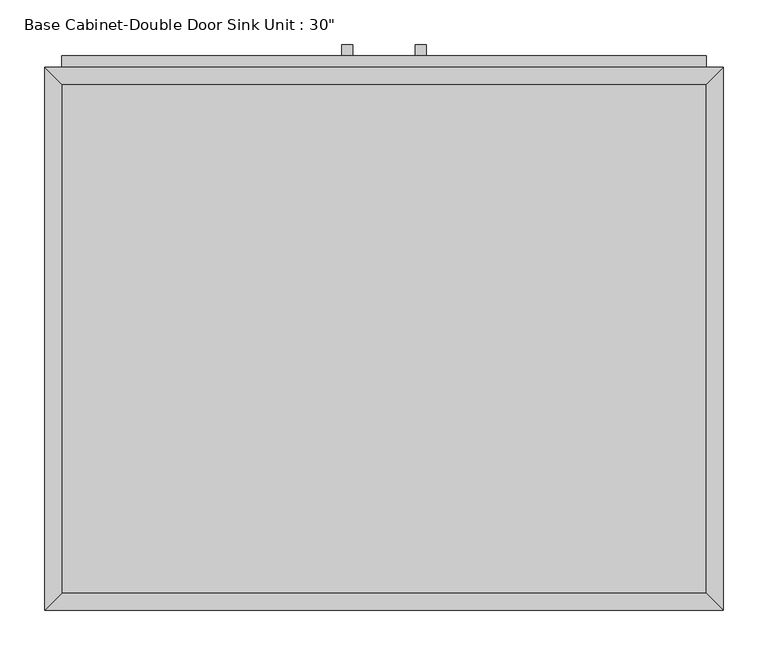
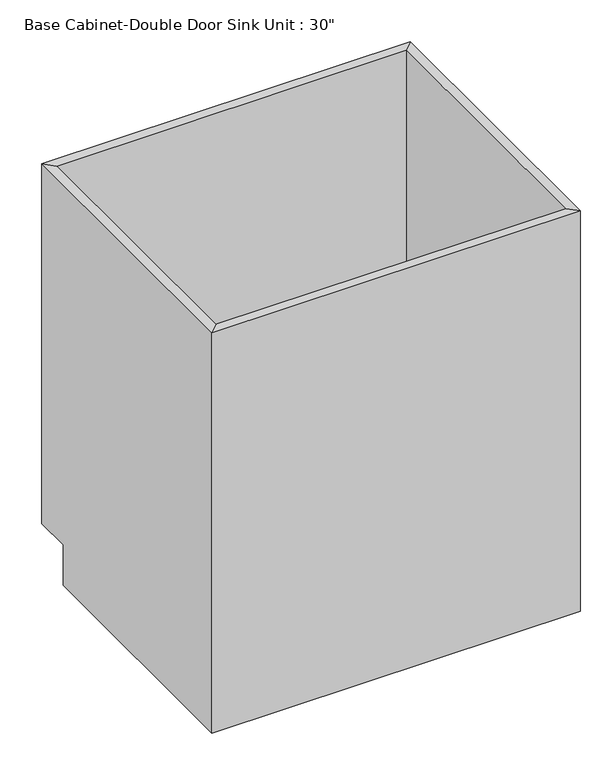
"""IFC4 building model written with IfcOpenShell, lengths in millimetres: furniture geometry."""

from ifc_helpers import new_model, si_unit, frame, origin, place, context, project, spatial, polyline, outline, extrude, faceted_brep, source, transform, mapped, element, save


def furniture_2feb49e6(model_context):
    return source(origin(), model_context, "Body", "SolidModel", [
        faceted_brep([(380.6877049, 590.55, 876.3), (-343.2122951, 590.55, 876.3), (-343.2122951, 590.55, 88.9), (380.6877049, 590.55, 88.9), (399.7377049, 609.6, 876.3), (-362.2622951, 609.6, 876.3), (399.7377049, 609.6, 88.9), (-362.2622951, 609.6, 88.9), (-343.2122951, 19.05, 876.3), (-343.2122951, 19.05, 88.9), (-343.2122951, 533.4, 88.9), (-362.2622951, 0.0, 876.3), (-362.2622951, 533.4, 88.9), (-362.2622951, 533.4, 0.0), (-362.2622951, 0.0, 0.0), (380.6877049, 19.05, 876.3), (380.6877049, 19.05, 88.9), (399.7377049, 0.0, 876.3), (399.7377049, 0.0, 0.0), (380.6877049, 533.4, 88.9), (399.7377049, 533.4, 0.0), (399.7377049, 533.4, 88.9)], [[[0, 1, 2, 3]], [[0, 4, 5, 1]], [[4, 6, 7, 5]], [[2, 7, 6, 3]], [[1, 8, 9, 10, 2]], [[5, 11, 8, 1]], [[7, 12, 13, 14, 11, 5]], [[2, 10, 12, 7]], [[8, 15, 16, 9]], [[11, 17, 15, 8]], [[14, 18, 17, 11]], [[3, 19, 16, 15, 0]], [[0, 15, 17, 4]], [[4, 17, 18, 20, 21, 6]], [[6, 21, 19, 3]], [[10, 9, 16, 19]], [[18, 14, 13, 20]], [[13, 12, 10, 19, 21, 20]]]),
        extrude(outline(polyline([(-16.1872951, 635.0), (-16.1872951, 622.3), (-28.8872951, 622.3), (-28.8872951, 635.0), (-16.1872951, 635.0)])), frame((0.0, 0.0, 573.769895), z_axis=(0.0, 0.0, 1.0), x_axis=(1.0, 0.0, 0.0)), (0.0, 0.0, 1.0), 124.730105),
        extrude(outline(polyline([(66.3627049, 635.0), (66.3627049, 622.3), (53.6627049, 622.3), (53.6627049, 635.0), (66.3627049, 635.0)])), frame((0.0, 0.0, 573.769895), z_axis=(0.0, 0.0, 1.0), x_axis=(1.0, 0.0, 0.0)), (0.0, 0.0, 1.0), 124.730105),
        extrude(outline(polyline([(380.6877049, 19.05), (-343.2122951, 19.05), (-343.2122951, 590.55), (380.6877049, 590.55), (380.6877049, 19.05)])), frame((0.0, 0.0, 88.9), z_axis=(0.0, 0.0, 1.0), x_axis=(1.0, 0.0, 0.0)), (0.0, 0.0, 1.0), 19.05),
        extrude(outline(polyline([(9.2127049, 622.3), (9.2127049, 609.6), (-343.2122951, 609.6), (-343.2122951, 622.3), (9.2127049, 622.3)])), frame((0.0, 0.0, 107.95), z_axis=(0.0, 0.0, 1.0), x_axis=(1.0, 0.0, 0.0)), (0.0, 0.0, 1.0), 628.65),
        extrude(outline(polyline([(380.6877049, 622.3), (380.6877049, 609.6), (28.2627049, 609.6), (28.2627049, 622.3), (380.6877049, 622.3)])), frame((0.0, 0.0, 107.95), z_axis=(0.0, 0.0, 1.0), x_axis=(1.0, 0.0, 0.0)), (0.0, 0.0, 1.0), 628.65),
        extrude(outline(polyline([(380.6877049, 622.3), (380.6877049, 609.6), (-343.2122951, 609.6), (-343.2122951, 622.3), (380.6877049, 622.3)])), frame((0.0, 0.0, 755.65), z_axis=(0.0, 0.0, 1.0), x_axis=(1.0, 0.0, 0.0)), (0.0, 0.0, 1.0), 101.6),
    ])


if __name__ == "__main__":
    model = new_model("IFC4")
    model_context = context("Model", 3, world=origin())
    ifc_project = project(units=[si_unit("LENGTHUNIT", "METRE", prefix="MILLI")], contexts=[model_context])
    site = spatial("IfcSite", under=ifc_project)
    building = spatial("IfcBuilding", under=site)
    placement = place(None, origin())
    furniture_shape = furniture_2feb49e6(model_context)
    element("IfcFurniture", 1, ObjectType="Base Cabinet-Double Door Sink Unit : 30\"", at=placement, inside=building, context=model_context, shape_type="MappedRepresentation", body=[
        mapped(furniture_shape, transform((0.0, 0.0, 0.0), x_axis=(1.0, 0.0, 0.0), y_axis=(0.0, 1.0, 0.0), z_axis=(0.0, 0.0, 1.0))),
    ])
    save(model, "model.ifc")

# Revit data of these elements
# Type "Base Cabinet-Double Door Sink Unit : 30\""
#   Assembly Code = "C1030410"
#   Depth = 2' - 0"
#   Height = 2' - 10 1/2"
#   Toe Depth = 0' - 3"
#   Toe Height = 0' - 3 1/2"
#   Width = 2' - 6"
#   Cabinet Material = none
#   Door/Drawer Material = none
#   Handle Material = Cabinets - Handles
#   Default Elevation = 0
# Element 1 (IfcFurniture, "Base Cabinet-Double Door Sink Unit : 30\"")
#   Materials on its faces: "Cabinets", "Cabinets - Handles"
# Materials
#   "Cabinets - Handles": class "Metal", colour RGB 57 57 57, transparency 0
#   "Cabinets": colour RGB 249 249 249, transparency 0
